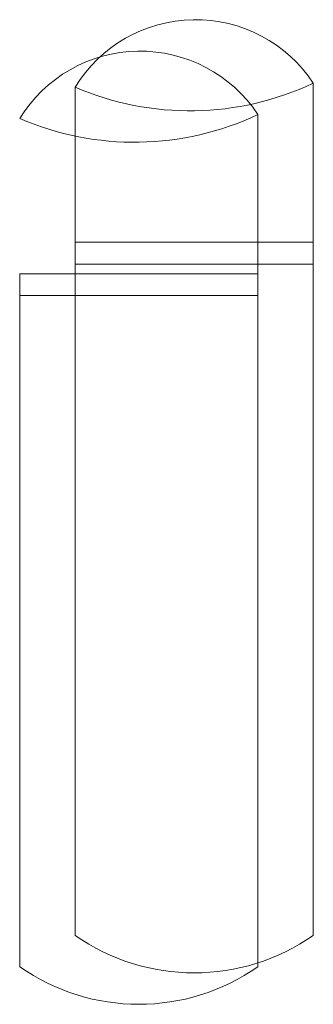
# Model space of a CAD drawing. Units: centimetres. Extents: x 5383 to 11288, y 5305 to 11515.
# Tile 5 of 5: x 11283.31 to 11287.63, y 11500.13 to 11514.63. Entities that reach past the tile are written whole.
import ezdxf

# ---------------------------------------------------------------- set-up
doc = ezdxf.new("R2010")
doc.units = ezdxf.units.CM
doc.layers.add('A-FURN-ACCS', color=9, linetype='Continuous', lineweight=13)

msp = doc.modelspace()

# ---------------------------------------------------------------- linework, layer by layer
at = {"layer": 'A-FURN-ACCS'}
for p, q in [((11287.629, 11511.352), (11287.629, 11513.696)), ((11284.126, 11511.352), (11284.126, 11513.639)), ((11286.814, 11510.889), (11286.814, 11513.233)), ((11284.126, 11511.352), (11284.126, 11501.143)), ((11284.126, 11511.352), (11287.629, 11511.352)), ((11287.629, 11511.352), (11287.629, 11501.143)), ((11284.126, 11511.032), (11287.629, 11511.032)), ((11283.312, 11510.889), (11283.312, 11500.68)), ((11283.312, 11510.889), (11286.814, 11510.889)), ((11286.814, 11510.889), (11286.814, 11500.68)), ((11283.312, 11510.569), (11286.814, 11510.569))]:
    msp.add_line(p, q, dxfattribs=at)
for centre, radius, start, end in [((11285.896, 11512.558), 2.073, 33.2806, 148.588), ((11285.081, 11512.095), 2.073, 33.2806, 148.588), ((11285.815, 11517.541), 4.252, 246.6072, 295.2614), ((11285, 11517.078), 4.252, 246.6072, 295.2614), ((11285.878, 11503.639), 3.049, 234.9464, 305.0536), ((11285.063, 11503.176), 3.049, 234.9464, 305.0536)]:
    msp.add_arc(centre, radius, start, end, dxfattribs=at)

doc.saveas('drawing.dxf')
